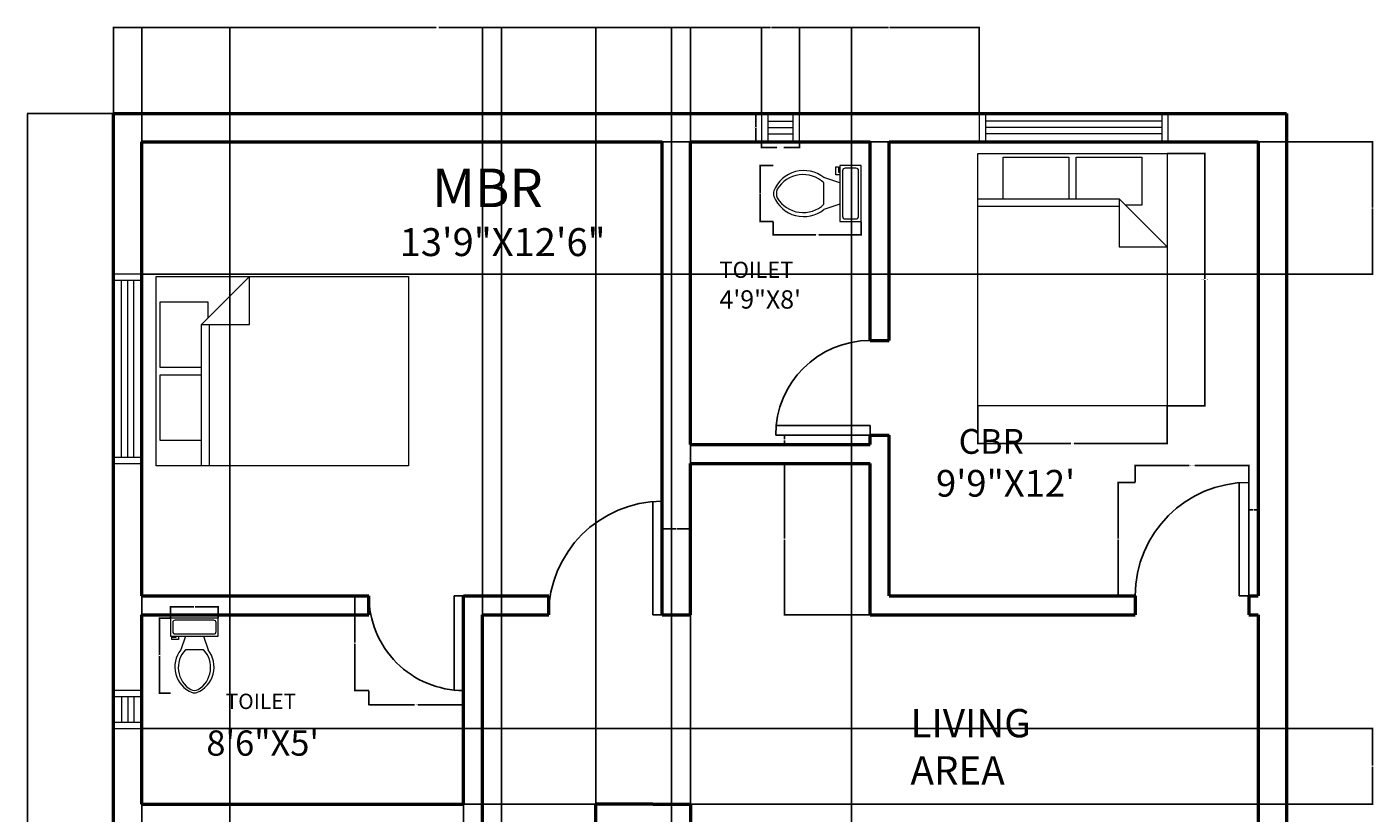
# Model space of a CAD drawing. Units: inches. Extents: x 16 to 443, y 39 to 637.
# Tile 3 of 3: x 16 to 443, y 387 to 637. Entities that reach past the tile are written whole.
import ezdxf

# ---------------------------------------------------------------- set-up
doc = ezdxf.new("R2010")
doc.units = ezdxf.units.IN
for name, color, linetype, lineweight in [('A-ANNO-DIMS', 2, 'Continuous', 18), ('A-AREA-IDEN', 7, 'Continuous', 18), ('A-DOOR', 3, 'Continuous', 25), ('A-FLOR-FIXT', 9, 'Continuous', 18), ('A-FURN', 8, 'Continuous', 18), ('A-GLAZ', 4, 'Continuous', 18), ('A-WALL', 7, 'Continuous', 50)]:
    doc.layers.add(name, color=color, linetype=linetype, lineweight=lineweight)
doc.styles.get("Standard").update_dxf_attribs({"font": 'arial.ttf'})
doc.dimstyles.get("Standard").update_dxf_attribs({"dimtxt": 0.18, "dimasz": 0.18, "dimexe": 0.18, "dimexo": 0.0625, "dimgap": 0.09, "dimtad": 0, "dimtih": 1, "dimtoh": 1, "dimdec": 4, "dimzin": 0, "dimdsep": 46, "dimtxsty": 'Standard', "dimcen": 0.09, "dimadec": 0, "dimazin": 0, "dimtfac": 1, "dimtdec": 4, "dimtofl": 0, "dimtmove": 0, "dimatfit": 3, "dimfxl": 1, "dimtolj": 1, "dimtzin": 0, "dimarcsym": 0})

# ---------------------------------------------------------------- blocks, each defined once
blk = doc.blocks.new('Bed - Queen')
for p, q in [((0, -80.00003), (0, 0)), ((0, 0), (59.99999, 0)), ((59.99999, 0), (59.99999, -80.00003)), ((7.99999, -1.2), (28.79998, -1.2)), ((7.99999, -14.4), (7.99999, -1.2)), ((28.79998, -1.2), (28.79998, -14.4)), ((31.19999, -1.2), (51.99999, -1.2)), ((31.19999, -14.4), (31.19999, -1.2)), ((51.99999, -1.2), (51.99999, -16.4)), ((0, -14.4), (44.8, -14.4)), ((44.8, -16.8), (0, -16.8)), ((59.99999, -29.6), (44.8, -14.4)), ((44.8, -14.4), (44.8, -29.6)), ((51.99999, -16.4), (46.79936, -16.4)), ((44.8, -29.6), (59.99999, -29.6)), ((59.99999, -80.00003), (0, -80.00003))]:
    blk.add_line(p, q)
blk = doc.blocks.new('Toilet - top')
for p, q in [((9.5, -6), (9.5, -2)), ((-10, -8.5), (-8, -8.5)), ((-10, -9.5), (-10, -8.5)), ((-7, -9.5), (-10, -9.5)), ((-8, -8.5), (-8, -8)), ((-7, -8), (-7, -9.5)), ((-4, -8), (-6, -14)), ((4, -8), (6, -14)), ((4, -14), (-4, -14))]:
    blk.add_line(p, q)
blk.add_lwpolyline([(10.5, -8), (10.5, 0), (-10.5, 0), (-10.5, -8)], close=True)
for points in [[(-9.5, -2), (-9.5, -6)], [(8.5, -1), (-8.5, -1)], [(-8.5, -7), (8.5, -7)]]:
    blk.add_lwpolyline(points)
for centre, radius, start, end in [((-8.62, -1.88), 0.884, 81.8699, 188.1301), ((8.62, -1.88), 0.884, 351.8699, 98.1301), ((-8.62, -6.12), 0.884, 171.8699, 278.1301), ((8.62, -6.12), 0.884, 261.8699, 8.1301), ((3.52, -21.58), 12.17, 141.4691, 247.9714), ((4.2, -21.82), 11.33, 136.3677, 238.9468), ((-3.52, -21.58), 12.17, 292.0284, 38.5307), ((-4.2, -21.82), 11.33, 301.053, 43.6321), ((0, -27.88), 4, 245.7318, 294.2682), ((0, -29), 4, 254.8605, 285.1395)]:
    blk.add_arc(centre, radius, start, end)
blk = doc.blocks.new('WIN-60IN')
for p, q in [((0, 60), (0, 0)), ((9, 60), (0, 60)), ((9, 0), (9, 60)), ((9, 58), (0, 58)), ((2.5, 58), (2.5, 2)), ((4.5, 58), (4.5, 2)), ((6.5, 58), (6.5, 2)), ((0, 2), (9, 2)), ((0, 0), (9, 0))]:
    blk.add_line(p, q)
blk = doc.blocks.new('WIN-12IN')
for p, q in [((0, 12), (0, 0)), ((9, 12), (0, 12)), ((9, 10), (0, 10)), ((2.5, 10), (2.5, 2)), ((4.5, 10), (4.5, 2)), ((6.5, 10), (6.5, 2)), ((9, 0), (9, 12)), ((0, 2), (9, 2)), ((0, 0), (9, 0))]:
    blk.add_line(p, q)
blk = doc.blocks.new('DOOR-SINGLE-36IN')
for p, q in [((33, 36), (33, 0)), ((36, 36), (36, 0)), ((36, 0), (33, 0))]:
    blk.add_line(p, q)
blk.add_arc((36, 0), 36, 90, 180)
blk = doc.blocks.new('DOOR-SINGLE-30IN')
for p, q in [((0, 3), (30, 3)), ((0, 0), (30, 0)), ((30, 0), (30, 3))]:
    blk.add_line(p, q)
blk.add_arc((30, 0), 30, 90, 180)
blk = doc.blocks.new('*D17')
at = {"layer": 'A-ANNO-DIMS', "color": 0, "lineweight": -2, "transparency": 16777216}
for p, q in [((249.25, 600.02), (249.25, 598.1)), ((249.43, 598.28), (254.13, 598.28)), ((261.07, 598.28), (256.37, 598.28)), ((261.25, 600.02), (261.25, 598.1))]:
    blk.add_line(p, q, dxfattribs=at)
at = {"layer": 'A-ANNO-DIMS', "color": 0, "transparency": 16777216}
for points in [[(249.43, 598.31), (249.43, 598.25), (249.25, 598.28)], [(261.07, 598.31), (261.07, 598.25), (261.25, 598.28)]]:
    blk.add_solid(points, dxfattribs=at)
at = {"layer": 'Defpoints', "color": 0, "transparency": 16777216}
for p in [(249.25, 600.08), (249.25, 598.28), (261.25, 600.08)]:
    blk.add_point(p, dxfattribs=at)
at = {"layer": 'A-ANNO-DIMS', "color": 0, "transparency": 16777216, "insert": (255.25, 598.28), "char_height": 0.18, "attachment_point": 5}
blk.add_mtext('\\A1;WINDOW 12 TYP.', dxfattribs=at)
blk = doc.blocks.new('*D18')
at = {"layer": 'A-ANNO-DIMS', "color": 0, "lineweight": -2, "transparency": 16777216}
for p, q in [((249.19, 609.08), (247.27, 609.08)), ((247.45, 608.9), (247.45, 604.76)), ((247.45, 600.26), (247.45, 604.4)), ((249.19, 600.08), (247.27, 600.08))]:
    blk.add_line(p, q, dxfattribs=at)
at = {"layer": 'A-ANNO-DIMS', "color": 0, "transparency": 16777216}
for points in [[(247.42, 608.9), (247.48, 608.9), (247.45, 609.08)], [(247.42, 600.26), (247.48, 600.26), (247.45, 600.08)]]:
    blk.add_solid(points, dxfattribs=at)
at = {"layer": 'Defpoints', "color": 0, "transparency": 16777216}
for p in [(247.45, 609.08), (249.25, 609.08), (249.25, 600.08)]:
    blk.add_point(p, dxfattribs=at)
at = {"layer": 'A-ANNO-DIMS', "color": 0, "transparency": 16777216, "insert": (247.45, 604.58), "char_height": 0.18, "attachment_point": 5}
blk.add_mtext('\\A1;9 TYP.', dxfattribs=at)
blk = doc.blocks.new('*D19')
at = {"layer": 'A-ANNO-DIMS', "color": 0, "lineweight": -2, "transparency": 16777216}
for p, q in [((367.75, 492.14), (367.75, 497.66)), ((367.93, 497.48), (384.81, 497.48)), ((403.57, 497.48), (386.68, 497.48)), ((403.75, 492.14), (403.75, 497.66))]:
    blk.add_line(p, q, dxfattribs=at)
at = {"layer": 'A-ANNO-DIMS', "color": 0, "transparency": 16777216}
for points in [[(367.93, 497.51), (367.93, 497.45), (367.75, 497.48)], [(403.57, 497.51), (403.57, 497.45), (403.75, 497.48)]]:
    blk.add_solid(points, dxfattribs=at)
at = {"layer": 'Defpoints', "color": 0, "transparency": 16777216}
for p in [(403.75, 497.48), (367.75, 492.08), (403.75, 492.08)]:
    blk.add_point(p, dxfattribs=at)
at = {"layer": 'A-ANNO-DIMS', "color": 0, "transparency": 16777216, "insert": (385.75, 497.48), "char_height": 0.18, "attachment_point": 5}
blk.add_mtext('\\A1;DOOR 36 TYP.', dxfattribs=at)
blk = doc.blocks.new('*D20')
at = {"layer": 'A-ANNO-DIMS', "color": 0, "lineweight": -2, "transparency": 16777216}
for p, q in [((367.69, 492.08), (362.17, 492.08)), ((362.35, 491.9), (362.35, 474.26)), ((362.35, 456.26), (362.35, 473.9)), ((367.69, 456.08), (362.17, 456.08))]:
    blk.add_line(p, q, dxfattribs=at)
at = {"layer": 'A-ANNO-DIMS', "color": 0, "transparency": 16777216}
for points in [[(362.32, 491.9), (362.38, 491.9), (362.35, 492.08)], [(362.32, 456.26), (362.38, 456.26), (362.35, 456.08)]]:
    blk.add_solid(points, dxfattribs=at)
at = {"layer": 'Defpoints', "color": 0, "transparency": 16777216}
for p in [(362.35, 492.08), (367.75, 492.08), (367.75, 456.08)]:
    blk.add_point(p, dxfattribs=at)
at = {"layer": 'A-ANNO-DIMS', "color": 0, "transparency": 16777216, "insert": (362.35, 474.08), "char_height": 0.18, "attachment_point": 5}
blk.add_mtext('\\A1;36 TYP.', dxfattribs=at)
blk = doc.blocks.new('*D21')
at = {"layer": 'A-ANNO-DIMS', "color": 0, "lineweight": -2, "transparency": 16777216}
for p, q in [((124.69, 456.08), (120.07, 456.08)), ((120.25, 455.9), (120.25, 441.26)), ((120.25, 426.26), (120.25, 440.9)), ((124.69, 426.08), (120.07, 426.08))]:
    blk.add_line(p, q, dxfattribs=at)
at = {"layer": 'A-ANNO-DIMS', "color": 0, "transparency": 16777216}
for points in [[(120.22, 455.9), (120.28, 455.9), (120.25, 456.08)], [(120.22, 426.26), (120.28, 426.26), (120.25, 426.08)]]:
    blk.add_solid(points, dxfattribs=at)
at = {"layer": 'Defpoints', "color": 0, "transparency": 16777216}
for p in [(120.25, 456.08), (124.75, 456.08), (124.75, 426.08)]:
    blk.add_point(p, dxfattribs=at)
at = {"layer": 'A-ANNO-DIMS', "color": 0, "transparency": 16777216, "insert": (120.25, 441.08), "char_height": 0.18, "attachment_point": 5}
blk.add_mtext('\\A1;DOOR 30 TYP.', dxfattribs=at)
blk = doc.blocks.new('*D22')
at = {"layer": 'A-ANNO-DIMS', "color": 0, "lineweight": -2, "transparency": 16777216}
for p, q in [((124.75, 426.02), (124.75, 421.4)), ((154.75, 426.02), (154.75, 421.4)), ((124.93, 421.58), (139.22, 421.58)), ((154.57, 421.58), (140.28, 421.58))]:
    blk.add_line(p, q, dxfattribs=at)
at = {"layer": 'A-ANNO-DIMS', "color": 0, "transparency": 16777216}
for points in [[(124.93, 421.61), (124.93, 421.55), (124.75, 421.58)], [(154.57, 421.61), (154.57, 421.55), (154.75, 421.58)]]:
    blk.add_solid(points, dxfattribs=at)
at = {"layer": 'Defpoints', "color": 0, "transparency": 16777216}
for p in [(124.75, 426.08), (154.75, 426.08), (124.75, 421.58)]:
    blk.add_point(p, dxfattribs=at)
at = {"layer": 'A-ANNO-DIMS', "color": 0, "transparency": 16777216, "insert": (139.75, 421.58), "char_height": 0.18, "attachment_point": 5}
blk.add_mtext('\\A1;30 TYP.', dxfattribs=at)
blk = doc.blocks.new('*D23')
at = {"layer": 'A-ANNO-DIMS', "color": 0, "lineweight": -2, "transparency": 16777216}
for p, q in [((377.92, 596.4), (390.03, 596.4)), ((389.85, 596.22), (389.85, 556.59)), ((389.85, 516.58), (389.85, 556.21)), ((377.92, 516.4), (390.03, 516.4))]:
    blk.add_line(p, q, dxfattribs=at)
at = {"layer": 'A-ANNO-DIMS', "color": 0, "transparency": 16777216}
for points in [[(389.82, 596.22), (389.88, 596.22), (389.85, 596.4)], [(389.82, 516.58), (389.88, 516.58), (389.85, 516.4)]]:
    blk.add_solid(points, dxfattribs=at)
at = {"layer": 'Defpoints', "color": 0, "transparency": 16777216}
for p in [(377.85, 596.4), (389.85, 596.4), (377.85, 516.4)]:
    blk.add_point(p, dxfattribs=at)
at = {"layer": 'A-ANNO-DIMS', "color": 0, "transparency": 16777216, "insert": (389.85, 556.4), "char_height": 0.18, "attachment_point": 5}
blk.add_mtext('\\A1;QUEEN BED 80 TYP.', dxfattribs=at)
blk = doc.blocks.new('*D24')
at = {"layer": 'A-ANNO-DIMS', "color": 0, "lineweight": -2, "transparency": 16777216}
for p, q in [((317.85, 516.34), (317.85, 504.22)), ((377.85, 516.34), (377.85, 504.22)), ((318.03, 504.4), (347.32, 504.4)), ((377.67, 504.4), (348.38, 504.4))]:
    blk.add_line(p, q, dxfattribs=at)
at = {"layer": 'A-ANNO-DIMS', "color": 0, "transparency": 16777216}
for points in [[(318.03, 504.43), (318.03, 504.37), (317.85, 504.4)], [(377.67, 504.43), (377.67, 504.37), (377.85, 504.4)]]:
    blk.add_solid(points, dxfattribs=at)
at = {"layer": 'Defpoints', "color": 0, "transparency": 16777216}
for p in [(317.85, 516.4), (377.85, 516.4), (377.85, 504.4)]:
    blk.add_point(p, dxfattribs=at)
at = {"layer": 'A-ANNO-DIMS', "color": 0, "transparency": 16777216, "insert": (347.85, 504.4), "char_height": 0.18, "attachment_point": 5}
blk.add_mtext('\\A1;60 TYP.', dxfattribs=at)
blk = doc.blocks.new('*D25')
at = {"layer": 'A-ANNO-DIMS', "color": 0, "lineweight": -2, "transparency": 16777216}
for p, q in [((61.8, 449.07), (58.11, 449.07)), ((58.29, 448.89), (58.29, 437.35)), ((58.29, 425.45), (58.29, 436.99)), ((61.8, 425.27), (58.11, 425.27))]:
    blk.add_line(p, q, dxfattribs=at)
at = {"layer": 'A-ANNO-DIMS', "color": 0, "transparency": 16777216}
for points in [[(58.26, 448.89), (58.32, 448.89), (58.29, 449.07)], [(58.26, 425.45), (58.32, 425.45), (58.29, 425.27)]]:
    blk.add_solid(points, dxfattribs=at)
at = {"layer": 'Defpoints', "color": 0, "transparency": 16777216}
for p in [(58.29, 449.07), (61.86, 449.07), (61.86, 425.27)]:
    blk.add_point(p, dxfattribs=at)
at = {"layer": 'A-ANNO-DIMS', "color": 0, "transparency": 16777216, "insert": (58.29, 437.17), "char_height": 0.18, "attachment_point": 5}
blk.add_mtext('\\A1;WC 24', dxfattribs=at)
blk = doc.blocks.new('*D26')
at = {"layer": 'A-ANNO-DIMS', "color": 0, "lineweight": -2, "transparency": 16777216}
for p, q in [((61.86, 449.13), (61.86, 452.81)), ((62.04, 452.63), (69.21, 452.63)), ((76.8, 452.63), (69.63, 452.63)), ((76.98, 449.13), (76.98, 452.81))]:
    blk.add_line(p, q, dxfattribs=at)
at = {"layer": 'A-ANNO-DIMS', "color": 0, "transparency": 16777216}
for points in [[(62.04, 452.66), (62.04, 452.6), (61.86, 452.63)], [(76.8, 452.66), (76.8, 452.6), (76.98, 452.63)]]:
    blk.add_solid(points, dxfattribs=at)
at = {"layer": 'Defpoints', "color": 0, "transparency": 16777216}
for p in [(76.98, 452.63), (61.86, 449.07), (76.98, 449.07)]:
    blk.add_point(p, dxfattribs=at)
at = {"layer": 'A-ANNO-DIMS', "color": 0, "transparency": 16777216, "insert": (69.42, 452.63), "char_height": 0.18, "attachment_point": 5}
blk.add_mtext('\\A1;15', dxfattribs=at)
blk = doc.blocks.new('*D27')
at = {"layer": 'A-ANNO-DIMS', "color": 0, "lineweight": -2, "transparency": 16777216}
for p, q in [((252.97, 574.73), (252.97, 570.42)), ((280.88, 574.73), (280.88, 570.42)), ((253.15, 570.6), (266.45, 570.6)), ((280.7, 570.6), (267.39, 570.6))]:
    blk.add_line(p, q, dxfattribs=at)
at = {"layer": 'A-ANNO-DIMS', "color": 0, "transparency": 16777216}
for points in [[(253.15, 570.63), (253.15, 570.57), (252.97, 570.6)], [(280.7, 570.63), (280.7, 570.57), (280.88, 570.6)]]:
    blk.add_solid(points, dxfattribs=at)
at = {"layer": 'Defpoints', "color": 0, "transparency": 16777216}
for p in [(252.97, 574.79), (280.88, 574.79), (280.88, 570.6)]:
    blk.add_point(p, dxfattribs=at)
at = {"layer": 'A-ANNO-DIMS', "color": 0, "transparency": 16777216, "insert": (266.92, 570.6), "char_height": 0.18, "attachment_point": 5}
blk.add_mtext('\\A1;WC 28', dxfattribs=at)
blk = doc.blocks.new('*D28')
at = {"layer": 'A-ANNO-DIMS', "color": 0, "lineweight": -2, "transparency": 16777216}
for p, q in [((252.9, 592.53), (248.6, 592.53)), ((248.78, 592.35), (248.78, 583.84)), ((248.78, 574.97), (248.78, 583.47)), ((252.9, 574.79), (248.6, 574.79))]:
    blk.add_line(p, q, dxfattribs=at)
at = {"layer": 'A-ANNO-DIMS', "color": 0, "transparency": 16777216}
for points in [[(248.75, 592.35), (248.81, 592.35), (248.78, 592.53)], [(248.75, 574.97), (248.81, 574.97), (248.78, 574.79)]]:
    blk.add_solid(points, dxfattribs=at)
at = {"layer": 'Defpoints', "color": 0, "transparency": 16777216}
for p in [(252.97, 592.53), (248.78, 574.79), (252.97, 574.79)]:
    blk.add_point(p, dxfattribs=at)
at = {"layer": 'A-ANNO-DIMS', "color": 0, "transparency": 16777216, "insert": (248.78, 583.66), "char_height": 0.18, "attachment_point": 5}
blk.add_mtext('\\A1;18', dxfattribs=at)
blk = doc.blocks.new('*D46')
at = {"layer": 'A-ANNO-DIMS', "color": 0, "lineweight": -2, "transparency": 16777216}
for p, q in [((43.69, 609.08), (16.32, 609.08)), ((16.5, 608.9), (16.5, 337.76)), ((16.5, 66.26), (16.5, 337.4)), ((277.69, 66.08), (16.32, 66.08))]:
    blk.add_line(p, q, dxfattribs=at)
at = {"layer": 'A-ANNO-DIMS', "color": 0, "transparency": 16777216}
for points in [[(16.47, 608.9), (16.53, 608.9), (16.5, 609.08)], [(16.47, 66.26), (16.53, 66.26), (16.5, 66.08)]]:
    blk.add_solid(points, dxfattribs=at)
at = {"layer": 'Defpoints', "color": 0, "transparency": 16777216}
for p in [(16.5, 609.08), (43.75, 609.08), (277.75, 66.08)]:
    blk.add_point(p, dxfattribs=at)
at = {"layer": 'A-ANNO-DIMS', "color": 0, "transparency": 16777216, "insert": (16.5, 337.58), "char_height": 0.18, "attachment_point": 5}
blk.add_mtext('\\A1;543', dxfattribs=at)
blk = doc.blocks.new('*D49')
at = {"layer": 'A-ANNO-DIMS', "color": 0, "lineweight": -2, "transparency": 16777216}
for p, q in [((226.75, 165.14), (226.75, 636.51)), ((226.93, 636.33), (252.05, 636.33)), ((277.57, 636.33), (252.45, 636.33)), ((277.75, 175.14), (277.75, 636.51))]:
    blk.add_line(p, q, dxfattribs=at)
at = {"layer": 'A-ANNO-DIMS', "color": 0, "transparency": 16777216}
for points in [[(226.93, 636.36), (226.93, 636.3), (226.75, 636.33)], [(277.57, 636.36), (277.57, 636.3), (277.75, 636.33)]]:
    blk.add_solid(points, dxfattribs=at)
at = {"layer": 'Defpoints', "color": 0, "transparency": 16777216}
for p in [(277.75, 636.33), (277.75, 175.08), (226.75, 165.08)]:
    blk.add_point(p, dxfattribs=at)
at = {"layer": 'A-ANNO-DIMS', "color": 0, "transparency": 16777216, "insert": (252.25, 636.33), "char_height": 0.18, "attachment_point": 5}
blk.add_mtext('\\A1;51', dxfattribs=at)
blk = doc.blocks.new('*D52')
at = {"layer": 'A-ANNO-DIMS', "color": 0, "lineweight": -2, "transparency": 16777216}
for p, q in [((43.75, 609.14), (43.75, 636.51)), ((43.93, 636.33), (146.1, 636.33)), ((249.07, 636.33), (146.9, 636.33)), ((249.25, 609.14), (249.25, 636.51))]:
    blk.add_line(p, q, dxfattribs=at)
at = {"layer": 'A-ANNO-DIMS', "color": 0, "transparency": 16777216}
for points in [[(43.93, 636.36), (43.93, 636.3), (43.75, 636.33)], [(249.07, 636.36), (249.07, 636.3), (249.25, 636.33)]]:
    blk.add_solid(points, dxfattribs=at)
at = {"layer": 'Defpoints', "color": 0, "transparency": 16777216}
for p in [(249.25, 636.33), (43.75, 609.08), (249.25, 609.08)]:
    blk.add_point(p, dxfattribs=at)
at = {"layer": 'A-ANNO-DIMS', "color": 0, "transparency": 16777216, "insert": (146.5, 636.33), "char_height": 0.18, "attachment_point": 5}
blk.add_mtext('\\A1;205.5', dxfattribs=at)
blk = doc.blocks.new('*D53')
at = {"layer": 'A-ANNO-DIMS', "color": 0, "lineweight": -2, "transparency": 16777216}
for p, q in [((261.25, 609.14), (261.25, 636.51)), ((261.43, 636.33), (289.53, 636.33)), ((318.07, 636.33), (289.97, 636.33)), ((318.25, 609.14), (318.25, 636.51))]:
    blk.add_line(p, q, dxfattribs=at)
at = {"layer": 'A-ANNO-DIMS', "color": 0, "transparency": 16777216}
for points in [[(261.43, 636.36), (261.43, 636.3), (261.25, 636.33)], [(318.07, 636.36), (318.07, 636.3), (318.25, 636.33)]]:
    blk.add_solid(points, dxfattribs=at)
at = {"layer": 'Defpoints', "color": 0, "transparency": 16777216}
for p in [(261.25, 636.33), (261.25, 609.08), (318.25, 609.08)]:
    blk.add_point(p, dxfattribs=at)
at = {"layer": 'A-ANNO-DIMS', "color": 0, "transparency": 16777216, "insert": (289.75, 636.33), "char_height": 0.18, "attachment_point": 5}
blk.add_mtext('\\A1;57', dxfattribs=at)
blk = doc.blocks.new('*D54')
at = {"layer": 'A-ANNO-DIMS', "color": 0, "lineweight": -2, "transparency": 16777216}
for p, q in [((52.81, 600.08), (443.18, 600.08)), ((443, 599.9), (443, 579.26)), ((443, 558.26), (443, 578.9)), ((52.81, 558.08), (443.18, 558.08))]:
    blk.add_line(p, q, dxfattribs=at)
at = {"layer": 'A-ANNO-DIMS', "color": 0, "transparency": 16777216}
for points in [[(442.97, 599.9), (443.03, 599.9), (443, 600.08)], [(442.97, 558.26), (443.03, 558.26), (443, 558.08)]]:
    blk.add_solid(points, dxfattribs=at)
at = {"layer": 'Defpoints', "color": 0, "transparency": 16777216}
for p in [(52.75, 600.08), (52.75, 558.08), (443, 558.08)]:
    blk.add_point(p, dxfattribs=at)
at = {"layer": 'A-ANNO-DIMS', "color": 0, "transparency": 16777216, "insert": (443, 579.08), "char_height": 0.18, "attachment_point": 5}
blk.add_mtext('\\A1;42', dxfattribs=at)
blk = doc.blocks.new('*D55')
at = {"layer": 'A-ANNO-DIMS', "color": 0, "lineweight": -2, "transparency": 16777216}
for p, q in [((52.81, 414.08), (443.18, 414.08)), ((443, 413.9), (443, 402.26)), ((443, 390.26), (443, 401.9)), ((52.81, 390.08), (443.18, 390.08))]:
    blk.add_line(p, q, dxfattribs=at)
at = {"layer": 'A-ANNO-DIMS', "color": 0, "transparency": 16777216}
for points in [[(442.97, 413.9), (443.03, 413.9), (443, 414.08)], [(442.97, 390.26), (443.03, 390.26), (443, 390.08)]]:
    blk.add_solid(points, dxfattribs=at)
at = {"layer": 'Defpoints', "color": 0, "transparency": 16777216}
for p in [(52.75, 414.08), (443, 414.08), (52.75, 390.08)]:
    blk.add_point(p, dxfattribs=at)
at = {"layer": 'A-ANNO-DIMS', "color": 0, "transparency": 16777216, "insert": (443, 402.08), "char_height": 0.18, "attachment_point": 5}
blk.add_mtext('\\A1;24', dxfattribs=at)
blk = doc.blocks.new('*D58')
at = {"layer": 'A-ANNO-DIMS', "color": 0, "lineweight": -2, "transparency": 16777216}
for p, q in [((160.75, 384.14), (160.75, 636.51)), ((160.93, 636.33), (178.53, 636.33)), ((196.57, 636.33), (178.97, 636.33)), ((196.75, 390.14), (196.75, 636.51))]:
    blk.add_line(p, q, dxfattribs=at)
at = {"layer": 'A-ANNO-DIMS', "color": 0, "transparency": 16777216}
for points in [[(160.93, 636.36), (160.93, 636.3), (160.75, 636.33)], [(196.57, 636.36), (196.57, 636.3), (196.75, 636.33)]]:
    blk.add_solid(points, dxfattribs=at)
at = {"layer": 'Defpoints', "color": 0, "transparency": 16777216}
for p in [(196.75, 636.33), (196.75, 390.08), (160.75, 384.08)]:
    blk.add_point(p, dxfattribs=at)
at = {"layer": 'A-ANNO-DIMS', "color": 0, "transparency": 16777216, "insert": (178.75, 636.33), "char_height": 0.18, "attachment_point": 5}
blk.add_mtext('\\A1;36', dxfattribs=at)
blk = doc.blocks.new('*D59')
at = {"layer": 'A-ANNO-DIMS', "color": 0, "lineweight": -2, "transparency": 16777216}
for p, q in [((154.75, 390.02), (154.75, 38.65)), ((160.75, 384.02), (160.75, 38.65)), ((154.93, 38.83), (157.6, 38.83)), ((160.57, 38.83), (157.9, 38.83))]:
    blk.add_line(p, q, dxfattribs=at)
at = {"layer": 'A-ANNO-DIMS', "color": 0, "transparency": 16777216}
for points in [[(154.93, 38.86), (154.93, 38.8), (154.75, 38.83)], [(160.57, 38.86), (160.57, 38.8), (160.75, 38.83)]]:
    blk.add_solid(points, dxfattribs=at)
at = {"layer": 'Defpoints', "color": 0, "transparency": 16777216}
for p in [(154.75, 390.08), (160.75, 384.08), (154.75, 38.83)]:
    blk.add_point(p, dxfattribs=at)
at = {"layer": 'A-ANNO-DIMS', "color": 0, "transparency": 16777216, "insert": (157.75, 38.83), "char_height": 0.18, "attachment_point": 5}
blk.add_mtext('\\A1;6', dxfattribs=at)
blk = doc.blocks.new('*D60')
at = {"layer": 'A-ANNO-DIMS', "color": 0, "lineweight": -2, "transparency": 16777216}
for p, q in [((166.75, 165.14), (166.75, 636.51)), ((166.93, 636.33), (193.53, 636.33)), ((220.57, 636.33), (193.97, 636.33)), ((220.75, 165.14), (220.75, 636.51))]:
    blk.add_line(p, q, dxfattribs=at)
at = {"layer": 'A-ANNO-DIMS', "color": 0, "transparency": 16777216}
for points in [[(166.93, 636.36), (166.93, 636.3), (166.75, 636.33)], [(220.57, 636.36), (220.57, 636.3), (220.75, 636.33)]]:
    blk.add_solid(points, dxfattribs=at)
at = {"layer": 'Defpoints', "color": 0, "transparency": 16777216}
for p in [(220.75, 636.33), (166.75, 165.08), (220.75, 165.08)]:
    blk.add_point(p, dxfattribs=at)
at = {"layer": 'A-ANNO-DIMS', "color": 0, "transparency": 16777216, "insert": (193.75, 636.33), "char_height": 0.18, "attachment_point": 5}
blk.add_mtext('\\A1;54', dxfattribs=at)
blk = doc.blocks.new('*D61')
at = {"layer": 'A-ANNO-DIMS', "color": 0, "lineweight": -2, "transparency": 16777216}
for p, q in [((52.75, 174.14), (52.75, 636.51)), ((52.93, 636.33), (66.23, 636.33)), ((80.47, 636.33), (67.16, 636.33)), ((80.65, 174.14), (80.65, 636.51))]:
    blk.add_line(p, q, dxfattribs=at)
at = {"layer": 'A-ANNO-DIMS', "color": 0, "transparency": 16777216}
for points in [[(52.93, 636.36), (52.93, 636.3), (52.75, 636.33)], [(80.47, 636.36), (80.47, 636.3), (80.65, 636.33)]]:
    blk.add_solid(points, dxfattribs=at)
at = {"layer": 'Defpoints', "color": 0, "transparency": 16777216}
for p in [(80.65, 636.33), (52.75, 174.08), (80.65, 174.08)]:
    blk.add_point(p, dxfattribs=at)
at = {"layer": 'A-ANNO-DIMS', "color": 0, "transparency": 16777216, "insert": (66.7, 636.33), "char_height": 0.18, "attachment_point": 5}
blk.add_mtext('\\A1;27.897', dxfattribs=at)
blk = doc.blocks.new('*D63')
at = {"layer": 'A-ANNO-DIMS', "color": 0, "lineweight": -2, "transparency": 16777216}
for p, q in [((403.75, 456.14), (403.75, 483.51)), ((403.93, 483.33), (405.1, 483.33)), ((406.57, 483.33), (405.4, 483.33)), ((406.75, 456.14), (406.75, 483.51))]:
    blk.add_line(p, q, dxfattribs=at)
at = {"layer": 'A-ANNO-DIMS', "color": 0, "transparency": 16777216}
for points in [[(403.93, 483.36), (403.93, 483.3), (403.75, 483.33)], [(406.57, 483.36), (406.57, 483.3), (406.75, 483.33)]]:
    blk.add_solid(points, dxfattribs=at)
at = {"layer": 'Defpoints', "color": 0, "transparency": 16777216}
for p in [(406.75, 483.33), (403.75, 456.08), (406.75, 456.08)]:
    blk.add_point(p, dxfattribs=at)
at = {"layer": 'A-ANNO-DIMS', "color": 0, "transparency": 16777216, "insert": (405.25, 483.33), "char_height": 0.18, "attachment_point": 5}
blk.add_mtext('\\A1;3', dxfattribs=at)
blk = doc.blocks.new('*D64')
at = {"layer": 'A-ANNO-DIMS', "color": 0, "lineweight": -2, "transparency": 16777216}
for p, q in [((283.69, 507.08), (256.32, 507.08)), ((283.69, 504.08), (256.32, 504.08)), ((256.5, 506.9), (256.5, 505.76)), ((256.5, 504.26), (256.5, 505.4))]:
    blk.add_line(p, q, dxfattribs=at)
at = {"layer": 'A-ANNO-DIMS', "color": 0, "transparency": 16777216}
for points in [[(256.47, 506.9), (256.53, 506.9), (256.5, 507.08)], [(256.47, 504.26), (256.53, 504.26), (256.5, 504.08)]]:
    blk.add_solid(points, dxfattribs=at)
at = {"layer": 'Defpoints', "color": 0, "transparency": 16777216}
for p in [(256.5, 507.08), (283.75, 507.08), (283.75, 504.08)]:
    blk.add_point(p, dxfattribs=at)
at = {"layer": 'A-ANNO-DIMS', "color": 0, "transparency": 16777216, "insert": (256.5, 505.58), "char_height": 0.18, "attachment_point": 5}
blk.add_mtext('\\A1;3', dxfattribs=at)
blk = doc.blocks.new('*D65')
at = {"layer": 'A-ANNO-DIMS', "color": 0, "lineweight": -2, "transparency": 16777216}
for p, q in [((217.75, 450.14), (217.75, 477.51)), ((217.93, 477.33), (222.1, 477.33)), ((226.57, 477.33), (222.4, 477.33)), ((226.75, 450.14), (226.75, 477.51))]:
    blk.add_line(p, q, dxfattribs=at)
at = {"layer": 'A-ANNO-DIMS', "color": 0, "transparency": 16777216}
for points in [[(217.93, 477.36), (217.93, 477.3), (217.75, 477.33)], [(226.57, 477.36), (226.57, 477.3), (226.75, 477.33)]]:
    blk.add_solid(points, dxfattribs=at)
at = {"layer": 'Defpoints', "color": 0, "transparency": 16777216}
for p in [(226.75, 477.33), (217.75, 450.08), (226.75, 450.08)]:
    blk.add_point(p, dxfattribs=at)
at = {"layer": 'A-ANNO-DIMS', "color": 0, "transparency": 16777216, "insert": (222.25, 477.33), "char_height": 0.18, "attachment_point": 5}
blk.add_mtext('\\A1;9', dxfattribs=at)
blk = doc.blocks.new('*D66')
at = {"layer": 'A-ANNO-DIMS', "color": 0, "lineweight": -2, "transparency": 16777216}
for p, q in [((283.69, 498.08), (256.32, 498.08)), ((256.5, 497.9), (256.5, 474.26)), ((256.5, 450.26), (256.5, 473.9)), ((283.69, 450.08), (256.32, 450.08))]:
    blk.add_line(p, q, dxfattribs=at)
at = {"layer": 'A-ANNO-DIMS', "color": 0, "transparency": 16777216}
for points in [[(256.47, 497.9), (256.53, 497.9), (256.5, 498.08)], [(256.47, 450.26), (256.53, 450.26), (256.5, 450.08)]]:
    blk.add_solid(points, dxfattribs=at)
at = {"layer": 'Defpoints', "color": 0, "transparency": 16777216}
for p in [(256.5, 498.08), (283.75, 498.08), (283.75, 450.08)]:
    blk.add_point(p, dxfattribs=at)
at = {"layer": 'A-ANNO-DIMS', "color": 0, "transparency": 16777216, "insert": (256.5, 474.08), "char_height": 0.18, "attachment_point": 5}
blk.add_mtext('\\A1;48', dxfattribs=at)

msp = doc.modelspace()

# ---------------------------------------------------------------- linework, layer by layer
at = {"layer": 'A-WALL'}
for p, q in [((43.7492, 165.0801), (43.7492, 609.0801)), ((43.7492, 609.0801), (415.7492, 609.0801)), ((415.7492, 609.0801), (415.7492, 66.0801)), ((52.7492, 600.0801), (217.7492, 600.0801)), ((52.7492, 456.0801), (52.7492, 600.0801)), ((217.7492, 450.0801), (217.7492, 600.0801)), ((226.7492, 600.0801), (283.7492, 600.0801)), ((226.7492, 504.0801), (226.7492, 600.0801)), ((283.7492, 537.0801), (283.7492, 600.0801)), ((289.7492, 600.0801), (406.7492, 600.0801)), ((289.7492, 537.0801), (289.7492, 600.0801)), ((406.7492, 600.0801), (406.7492, 456.0801)), ((283.7492, 537.0801), (289.7492, 537.0801)), ((226.7492, 504.0801), (283.7492, 504.0801)), ((283.7492, 507.0801), (289.7492, 507.0801)), ((283.7492, 504.0801), (283.7492, 507.0801)), ((289.7492, 456.0801), (289.7492, 507.0801)), ((226.7492, 450.0801), (226.7492, 498.0801)), ((226.7492, 498.0801), (283.7492, 498.0801)), ((283.7492, 450.0801), (283.7492, 498.0801)), ((52.7492, 456.0801), (124.7492, 456.0801)), ((124.7492, 450.0801), (124.7492, 456.0801)), ((154.7492, 390.0801), (154.7492, 456.0801)), ((154.7492, 456.0801), (181.7492, 456.0801)), ((181.7492, 450.0801), (181.7492, 456.0801)), ((289.7492, 456.0801), (367.7492, 456.0801)), ((367.7492, 456.0801), (367.7492, 450.0801)), ((403.7492, 456.0801), (403.7492, 450.0801)), ((403.7492, 456.0801), (406.7492, 456.0801)), ((52.7492, 450.0801), (124.7492, 450.0801)), ((52.7492, 390.0801), (52.7492, 450.0801)), ((160.7492, 384.0801), (160.7492, 450.0801)), ((160.7492, 450.0801), (181.7492, 450.0801)), ((217.7492, 450.0801), (226.7492, 450.0801)), ((283.7492, 450.0801), (367.7492, 450.0801)), ((403.7492, 450.0801), (406.7492, 450.0801)), ((406.7492, 450.0801), (406.7492, 175.0801)), ((52.7492, 390.0801), (154.7492, 390.0801)), ((214.7492, 390.0801), (196.7492, 390.0801)), ((196.7492, 384.0801), (196.7492, 390.0801)), ((214.7492, 390.0801), (226.7492, 390.0801)), ((226.7492, 390.0801), (226.7492, 165.0801))]:
    msp.add_line(p, q, dxfattribs=at)

# ---------------------------------------------------------------- block references
at = {"layer": 'A-DOOR'}
for name, p in [('DOOR-SINGLE-30IN', (253.749, 507.08)), ('DOOR-SINGLE-36IN', (367.749, 456.08)), ('DOOR-SINGLE-36IN', (181.749, 450.08))]:
    msp.add_blockref(name, p, dxfattribs=at)
at = {"layer": 'A-DOOR', "rotation": 90.0000000000001}
msp.add_blockref('DOOR-SINGLE-30IN', (154.7493, 426.0799), dxfattribs=at)
at = {"layer": 'A-FLOR-FIXT', "xscale": 0.8446766902417513, "yscale": 0.8446766902417513, "zscale": 0.8446766902417513, "rotation": 270}
msp.add_blockref('Toilet - top', (280.8784, 583.6568), dxfattribs=at)
at = {"layer": 'A-FLOR-FIXT', "xscale": 0.7199755172784759, "yscale": 0.7199755172784759, "zscale": 0.7199755172784759}
msp.add_blockref('Toilet - top', (69.4194, 449.0652), dxfattribs=at)
at = {"layer": 'A-FURN'}
msp.add_blockref('Bed - Queen', (317.8529, 596.3983), dxfattribs=at)
at = {"layer": 'A-FURN', "rotation": 90}
msp.add_blockref('Bed - Queen', (57.2957, 497.3505), dxfattribs=at)
at = {"layer": 'A-GLAZ'}
for name, p, rotation in [('WIN-12IN', (261.2493, 600.0799), 89.99999999999928), ('WIN-60IN', (318.2491, 609.0803), 269.9999999999999), ('WIN-60IN', (52.7494, 558.0802), 180)]:
    msp.add_blockref(name, p, dxfattribs=dict(at, rotation=rotation))
msp.add_blockref('WIN-12IN', (43.749, 414.08), dxfattribs=at)

# ---------------------------------------------------------------- texts
at = {"layer": 'A-AREA-IDEN', "attachment_point": 1}
for s, width, gutter_width, insert, char_height in [('MBR', 834.134541, 61.166, (144.7876, 591.5915), 12.23321), ('13\'9"X12\'6"', 603.461344, 44.2511, (134.5226, 572.6957), 8.850211), ('TOILET', 348.376212, 25.546, (235.9037, 562.0407), 5.1092), ('4\'9"X8\'', 395.412353, 28.9951, (235.9037, 552.9909), 5.79902), ('CBR', 535.872862, 39.2949, (311.7563, 508.9953), 7.85898), ('9\'9"X12\'', 576.923125, 42.305, (304.5876, 496.0208), 8.46101), ('TOILET', 331.871522, 24.3357, (79.3172, 425.0773), 4.86714), ('LIVING\\PAREA', 612.003404, 44.8774, (296.4907, 420.2115), 8.97549), ('8\'6"X5\'', 546.280856, 40.0581, (73.1971, 413.4215), 8.01162)]:
    msp.add_mtext_dynamic_manual_height_columns(s, width=width, gutter_width=gutter_width, heights=[0], dxfattribs=dict(at, insert=insert, char_height=char_height))

# ---------------------------------------------------------------- dimensions: what is measured, and where the dimension line sits
at = {"layer": 'A-ANNO-DIMS'}
for base, p1, p2, override, picture, middle in [((249.2492, 636.3301), (43.7492, 609.0801), (249.2492, 609.0801), {"dimdec": 1, "dimlfac": 1, "dimrnd": 0, "dimzin": 0, "dimdsep": 46, "dimlunit": 2}, '*D52', (146.4992, 636.3301)), ((80.6458, 636.3301), (52.7492, 174.0801), (80.6458, 174.0801), {"dimdec": 3, "dimlfac": 1, "dimrnd": 0, "dimzin": 0, "dimdsep": 46, "dimlunit": 2}, '*D61', (66.6975, 636.3301)), ((196.7492, 636.3301), (160.7492, 384.0801), (196.7492, 390.0801), {"dimdec": 0, "dimlfac": 1, "dimrnd": 0, "dimzin": 0, "dimdsep": 46, "dimlunit": 2}, '*D58', (178.7492, 636.3301)), ((220.7492, 636.3301), (166.7492, 165.0801), (220.7492, 165.0801), {"dimdec": 0, "dimlfac": 1, "dimrnd": 0, "dimzin": 0, "dimdsep": 46, "dimlunit": 2}, '*D60', (193.7492, 636.3301)), ((277.7492, 636.3301), (226.7492, 165.0801), (277.7492, 175.0801), {"dimdec": 0, "dimlfac": 1, "dimrnd": 0, "dimzin": 0, "dimdsep": 46, "dimlunit": 2}, '*D49', (252.2492, 636.3301)), ((261.2492, 636.3301), (318.2492, 609.0801), (261.2492, 609.0801), {"dimdec": 0, "dimlfac": 1, "dimrnd": 0, "dimzin": 0, "dimdsep": 46, "dimlunit": 2}, '*D53', (289.7492, 636.3301)), ((226.7492, 477.3301), (217.7492, 450.0801), (226.7492, 450.0801), {"dimdec": 0, "dimlfac": 1, "dimrnd": 0, "dimzin": 0, "dimdsep": 46, "dimlunit": 2}, '*D65', (222.2492, 477.3301)), ((76.9791, 452.634), (61.8596, 449.0652), (76.9791, 449.0652), {"dimdec": 0, "dimlfac": 1, "dimrnd": 0, "dimzin": 0, "dimdsep": 46, "dimlunit": 2}, '*D26', (69.4194, 452.634)), ((154.7492, 38.8301), (160.7492, 384.0801), (154.7492, 390.0801), {"dimdec": 0, "dimlfac": 1, "dimrnd": 0, "dimzin": 0, "dimdsep": 46, "dimlunit": 2}, '*D59', (157.7492, 38.8301))]:
    dim = msp.add_linear_dim(base=base, p1=p1, p2=p2, dimstyle='Standard', override=override, dxfattribs=at)
    dim.commit()
    dim.dimension.update_dxf_attribs({"geometry": picture, "text_midpoint": middle})
for base, p1, p2, angle, picture, middle in [((16.4992, 609.0801), (277.7492, 66.0801), (43.7492, 609.0801), 90, '*D46', (16.4992, 337.5801)), ((442.9992, 558.0801), (52.7492, 600.0801), (52.7492, 558.0801), 90, '*D54', (442.9992, 579.0801)), ((248.778, 574.7877), (252.965, 592.5259), (252.965, 574.7877), 270, '*D28', (248.778, 583.6568)), ((256.4992, 507.0801), (283.7492, 504.0801), (283.7492, 507.0801), 90, '*D64', (256.4992, 505.5801)), ((256.4992, 498.0801), (283.7492, 450.0801), (283.7492, 498.0801), 90, '*D66', (256.4992, 474.0801)), ((406.7492, 483.3301), (403.7492, 456.0801), (406.7492, 456.0801), 0, '*D63', (405.2492, 483.3301)), ((442.9992, 414.0801), (52.7492, 390.0801), (52.7492, 414.0801), 90, '*D55', (442.9992, 402.0801))]:
    dim = msp.add_linear_dim(base=base, p1=p1, p2=p2, angle=angle, dimstyle='Standard', override={"dimdec": 0, "dimlfac": 1, "dimrnd": 0, "dimzin": 0, "dimdsep": 46, "dimlunit": 2}, dxfattribs=at)
    dim.commit()
    dim.dimension.update_dxf_attribs({"geometry": picture, "text_midpoint": middle})
for base, p1, p2, angle, text, picture, middle in [((247.4492, 609.0801), (249.2492, 600.0801), (249.2492, 609.0801), 90, '<> TYP.', '*D18', (247.4492, 604.5801)), ((249.2492, 598.2801), (261.2492, 600.0801), (249.2492, 600.0801), 180, 'WINDOW <> TYP.', '*D17', (255.2492, 598.2801)), ((389.8529, 596.3983), (377.8529, 516.3983), (377.8529, 596.3983), 90, 'QUEEN BED <> TYP.', '*D23', (389.8529, 556.3983)), ((362.3492, 492.0801), (367.7492, 456.0801), (367.7492, 492.0801), 90, '<> TYP.', '*D20', (362.3492, 474.0801)), ((120.2492, 456.0801), (124.7492, 426.0801), (124.7492, 456.0801), 90, 'DOOR <> TYP.', '*D21', (120.2492, 441.0801)), ((58.2908, 449.0652), (61.8596, 425.2727), (61.8596, 449.0652), 90, 'WC <>', '*D25', (58.2908, 437.1689)), ((124.7492, 421.5801), (154.7492, 426.0801), (124.7492, 426.0801), 180, '<> TYP.', '*D22', (139.7492, 421.5801))]:
    dim = msp.add_linear_dim(base=base, p1=p1, p2=p2, angle=angle, text=text, dimstyle='Standard', override={"dimdec": 0, "dimlfac": 1, "dimrnd": 0, "dimzin": 0, "dimdsep": 46, "dimlunit": 2}, dxfattribs=at)
    dim.commit()
    dim.dimension.update_dxf_attribs({"geometry": picture, "text_midpoint": middle})
for base, p1, p2, text, picture, middle in [((280.8784, 570.6007), (252.965, 574.7877), (280.8784, 574.7877), 'WC <>', '*D27', (266.9217, 570.6007)), ((377.8529, 504.3983), (317.8529, 516.3983), (377.8529, 516.3983), '<> TYP.', '*D24', (347.8529, 504.3983)), ((403.7492, 497.4801), (367.7492, 492.0801), (403.7492, 492.0801), 'DOOR <> TYP.', '*D19', (385.7492, 497.4801))]:
    dim = msp.add_linear_dim(base=base, p1=p1, p2=p2, text=text, dimstyle='Standard', override={"dimdec": 0, "dimlfac": 1, "dimrnd": 0, "dimzin": 0, "dimdsep": 46, "dimlunit": 2}, dxfattribs=at)
    dim.commit()
    dim.dimension.update_dxf_attribs({"geometry": picture, "text_midpoint": middle})

doc.saveas('drawing.dxf')
